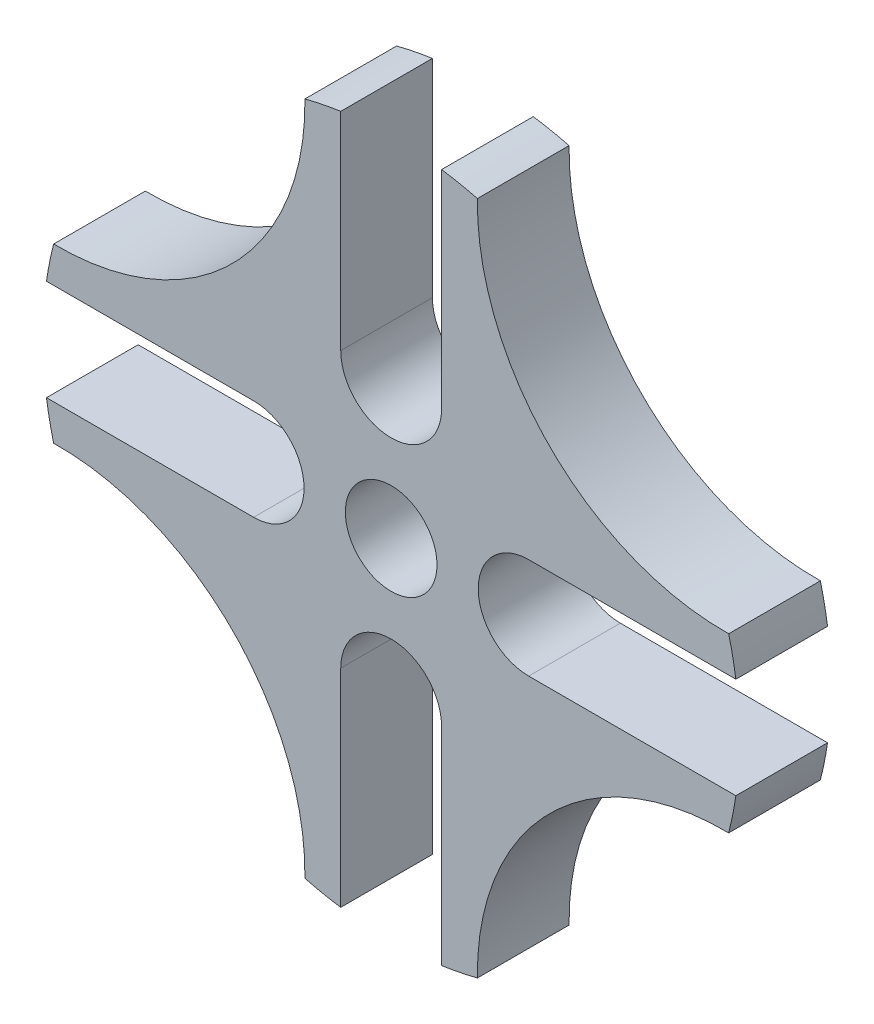
from build123d import *

# Parameters (mm, degrees)
SPIDER_PLATE_PROFILE_R          = 5
SPIDER_PLATE_EXTRUDE_10MM_DEPTH = 10


with BuildPart() as part:
    # Spider Plate Profile → Spider Plate Extrude 10mm (new body)
    with BuildSketch(Plane.XY):
        with BuildLine():
            Line((5.5, -15), (5.5, -37.599867021))
            ThreePointArc((5.5, -37.599867021), (7.46440512, -37.259665272), (9.408264389, -36.816905916))
            ThreePointArc((9.408264389, -36.816905916), (17.313241035, -17.313241035), (36.816905916, -9.408264389))
            ThreePointArc((36.816905916, -9.408264389), (37.259665272, -7.46440512), (37.599867021, -5.5))
            Line((37.599867021, -5.5), (15, -5.5))
            ThreePointArc((15, -5.5), (9.5, 0), (15, 5.5))
            Line((15, 5.5), (37.599867021, 5.5))
            ThreePointArc((37.599867021, 5.5), (37.259665272, 7.46440512), (36.816905916, 9.408264389))
            ThreePointArc((36.816905916, 9.408264389), (17.313241035, 17.313241035), (9.408264389, 36.816905916))
            ThreePointArc((9.408264389, 36.816905916), (7.46440512, 37.259665272), (5.5, 37.599867021))
            Line((5.5, 37.599867021), (5.5, 15))
            ThreePointArc((5.5, 15), (0, 9.5), (-5.5, 15))
            Line((-5.5, 15), (-5.5, 37.599867021))
            ThreePointArc((-5.5, 37.599867021), (-7.46440512, 37.259665272), (-9.408264389, 36.816905916))
            ThreePointArc((-9.408264389, 36.816905916), (-17.313241035, 17.313241035), (-36.816905916, 9.408264389))
            ThreePointArc((-36.816905916, 9.408264389), (-37.259665272, 7.46440512), (-37.599867021, 5.5))
            Line((-37.599867021, 5.5), (-15, 5.5))
            ThreePointArc((-15, 5.5), (-9.5, 0), (-15, -5.5))
            Line((-15, -5.5), (-37.599867021, -5.5))
            ThreePointArc((-37.599867021, -5.5), (-37.259665272, -7.46440512), (-36.816905916, -9.408264389))
            ThreePointArc((-36.816905916, -9.408264389), (-17.313241035, -17.313241035), (-9.408264389, -36.816905916))
            ThreePointArc((-9.408264389, -36.816905916), (-7.46440512, -37.259665272), (-5.5, -37.599867021))
            Line((-5.5, -37.599867021), (-5.5, -15))
            ThreePointArc((-5.5, -15), (0, -9.5), (5.5, -15))
        make_face()
        Circle(SPIDER_PLATE_PROFILE_R, mode=Mode.SUBTRACT)
    extrude(amount=SPIDER_PLATE_EXTRUDE_10MM_DEPTH)


solid = part.part
